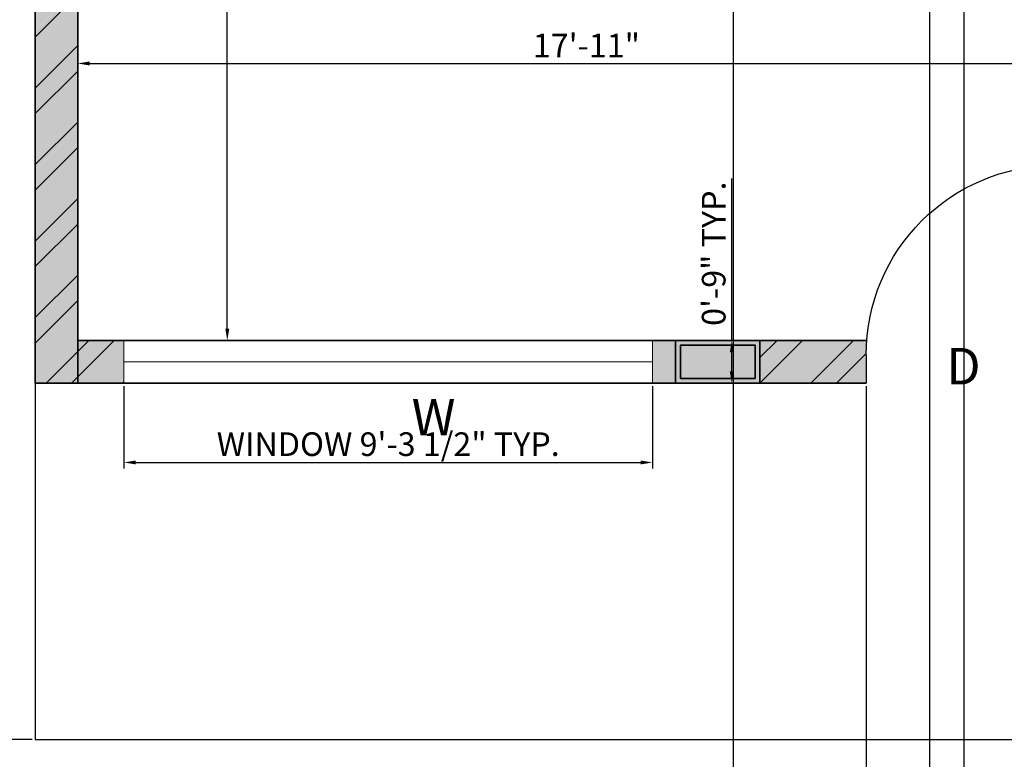
# Model space of a CAD drawing. Units: inches. Extents: x 1804 to 3296, y 909 to 2477.
# Tile 3 of 31: x 1922 to 2130, y 1059 to 1215. Entities that reach past the tile are written whole.
import ezdxf

# ---------------------------------------------------------------- set-up
doc = ezdxf.new("R2010")
doc.units = ezdxf.units.IN
for name, color, linetype, lineweight in [('A-ANNO-DIMS', 2, 'Continuous', 18), ('A-ANNO-TTLB', 156, 'Continuous', 35), ('A-WALL-PATT', 10, 'Continuous', 13), ('C-PROP', 7, 'Continuous', 25), ('DOOR', 30, 'Continuous', 25), ('TEXT', 190, 'Continuous', 18), ('WALL', 10, 'Continuous', 35), ('WIND', 130, 'Continuous', 18)]:
    doc.layers.add(name, color=color, linetype=linetype, lineweight=lineweight)
doc.styles.get("Standard").update_dxf_attribs({"font": 'arial.ttf'})
doc.dimstyles.new('ISO-25', dxfattribs={"dimtxt": 5, "dimasz": 2.5, "dimexe": 1.25, "dimexo": 0.625, "dimtad": 1, "dimdec": 0, "dimlunit": 4, "dimtxsty": 'Standard', "dimcen": 2.5, "dimadec": 0, "dimazin": 0, "dimtfac": 1, "dimtdec": 0, "dimtmove": 0, "dimatfit": 3, "dimfxl": 1, "dimarcsym": 0})

# ---------------------------------------------------------------- blocks, each defined once
blk = doc.blocks.new('*U2')
for p, q in [((0, 0), (0, -6)), ((40, 0), (40, -6))]:
    blk.add_line(p, q)
blk.add_lwpolyline([(0, 0), (0, 40), (1.75, 40), (1.75, 0)], close=True)
blk.add_arc((0, 0), 40, 0, 90)
blk = doc.blocks.new('*D21')
at = {"layer": 'A-ANNO-DIMS', "color": 0, "lineweight": -2, "transparency": 16777216}
for p, q in [((1935.21, 1539.88), (1967.44, 1539.88)), ((1966.19, 1149.57), (1966.19, 1537.38)), ((1935.21, 1147.07), (1967.44, 1147.07))]:
    blk.add_line(p, q, dxfattribs=at)
at = {"layer": 'A-ANNO-DIMS', "color": 0, "lineweight": 100, "transparency": 16777216}
for points in [[(1965.78, 1537.38), (1966.61, 1537.38), (1966.19, 1539.88)], [(1965.78, 1149.57), (1966.61, 1149.57), (1966.19, 1147.07)]]:
    blk.add_solid(points, dxfattribs=at)
at = {"layer": 'Defpoints', "color": 0, "lineweight": 100, "transparency": 16777216}
for p in [(1934.58, 1539.88), (1966.19, 1539.88), (1934.58, 1147.07)]:
    blk.add_point(p, dxfattribs=at)
at = {"layer": 'A-ANNO-DIMS', "color": 0, "transparency": 16777216, "insert": (1963.01, 1343.47), "char_height": 5, "attachment_point": 5, "rotation": 90}
blk.add_mtext('32\'-9"', dxfattribs=at)
blk = doc.blocks.new('*D22')
at = {"layer": 'A-ANNO-DIMS', "color": 0, "lineweight": -2, "transparency": 16777216}
for p, q in [((1934.58, 1147.69), (1934.58, 1206.88)), ((1937.08, 1205.63), (2147.08, 1205.63)), ((2149.58, 1147.69), (2149.58, 1206.88))]:
    blk.add_line(p, q, dxfattribs=at)
at = {"layer": 'A-ANNO-DIMS', "color": 0, "lineweight": 100, "transparency": 16777216}
for points in [[(1937.08, 1206.05), (1937.08, 1205.22), (1934.58, 1205.63)], [(2147.08, 1206.05), (2147.08, 1205.22), (2149.58, 1205.63)]]:
    blk.add_solid(points, dxfattribs=at)
at = {"layer": 'Defpoints', "color": 0, "lineweight": 100, "transparency": 16777216}
for p in [(2149.58, 1205.63), (1934.58, 1147.07), (2149.58, 1147.07)]:
    blk.add_point(p, dxfattribs=at)
at = {"layer": 'A-ANNO-DIMS', "color": 0, "transparency": 16777216, "insert": (2042.08, 1208.77), "char_height": 5, "attachment_point": 5}
blk.add_mtext('17\'-11"', dxfattribs=at)
blk = doc.blocks.new('WINDOW-PLAN-112IN')
blk.add_line((0, 4.5), (111.7, 4.5))
blk.add_lwpolyline([(0, 0), (111.7, 0), (111.7, 9), (0, 9)], close=True)
blk = doc.blocks.new('*D47')
at = {"layer": 'A-ANNO-DIMS', "color": 0, "lineweight": -2, "transparency": 16777216}
for p, q in [((1944.35, 1137.44), (1944.35, 1120.06)), ((2056.05, 1137.44), (2056.05, 1120.06)), ((1946.85, 1121.31), (2053.55, 1121.31))]:
    blk.add_line(p, q, dxfattribs=at)
at = {"layer": 'A-ANNO-DIMS', "color": 0, "lineweight": 100, "transparency": 16777216}
for points in [[(1946.85, 1121.73), (1946.85, 1120.9), (1944.35, 1121.31)], [(2053.55, 1121.73), (2053.55, 1120.9), (2056.05, 1121.31)]]:
    blk.add_solid(points, dxfattribs=at)
at = {"layer": 'Defpoints', "color": 0, "lineweight": 100, "transparency": 16777216}
for p in [(1944.35, 1138.07), (2056.05, 1138.07), (2056.05, 1121.31)]:
    blk.add_point(p, dxfattribs=at)
at = {"layer": 'A-ANNO-DIMS', "color": 0, "transparency": 16777216, "insert": (2000.2, 1124.53), "char_height": 5, "attachment_point": 5}
blk.add_mtext('WINDOW 9\'-3 1/2" TYP.', dxfattribs=at)
blk = doc.blocks.new('*D48')
at = {"layer": 'A-ANNO-DIMS', "color": 0, "lineweight": -2, "transparency": 16777216}
for p, q in [((2072.81, 1147.07), (2072.81, 1181.3)), ((2056.68, 1147.07), (2074.06, 1147.07)), ((2072.81, 1140.57), (2072.81, 1144.57)), ((2056.68, 1138.07), (2074.06, 1138.07))]:
    blk.add_line(p, q, dxfattribs=at)
at = {"layer": 'A-ANNO-DIMS', "color": 0, "lineweight": 100, "transparency": 16777216}
for points in [[(2072.39, 1144.57), (2073.22, 1144.57), (2072.81, 1147.07)], [(2072.39, 1140.57), (2073.22, 1140.57), (2072.81, 1138.07)]]:
    blk.add_solid(points, dxfattribs=at)
at = {"layer": 'Defpoints', "color": 0, "lineweight": 100, "transparency": 16777216}
for p in [(2056.05, 1147.07), (2072.81, 1147.07), (2056.05, 1138.07)]:
    blk.add_point(p, dxfattribs=at)
at = {"layer": 'A-ANNO-DIMS', "color": 0, "transparency": 16777216, "insert": (2069.63, 1165.43), "char_height": 5, "attachment_point": 5, "rotation": 90}
blk.add_mtext('0\'-9" TYP.', dxfattribs=at)
blk = doc.blocks.new('*D52')
at = {"layer": 'A-ANNO-DIMS', "color": 0, "lineweight": -2, "transparency": 16777216}
for p, q in [((1924.96, 1830.04), (1880.63, 1830.04)), ((1881.88, 1065.27), (1881.88, 1827.54)), ((1924.96, 1062.77), (1880.63, 1062.77))]:
    blk.add_line(p, q, dxfattribs=at)
at = {"layer": 'A-ANNO-DIMS', "color": 0, "lineweight": 100, "transparency": 16777216}
for points in [[(1881.47, 1827.54), (1882.3, 1827.54), (1881.88, 1830.04)], [(1881.47, 1065.27), (1882.3, 1065.27), (1881.88, 1062.77)]]:
    blk.add_solid(points, dxfattribs=at)
at = {"layer": 'Defpoints', "color": 0, "lineweight": 100, "transparency": 16777216}
for p in [(1881.88, 1830.04), (1925.58, 1830.04), (1925.58, 1062.77)]:
    blk.add_point(p, dxfattribs=at)
at = {"layer": 'A-ANNO-DIMS', "color": 0, "transparency": 16777216, "insert": (1878.67, 1446.4), "char_height": 5, "attachment_point": 5, "rotation": 90}
blk.add_mtext('63\'-11 1/2"', dxfattribs=at)
blk = doc.blocks.new('*D59')
at = {"layer": 'A-ANNO-DIMS', "color": 0, "lineweight": -2, "transparency": 16777216}
for p, q in [((2121.83, 1590.3), (2121.83, 975.89)), ((2161.83, 1590.3), (2161.83, 975.89)), ((2124.33, 977.14), (2159.33, 977.14))]:
    blk.add_line(p, q, dxfattribs=at)
at = {"layer": 'A-ANNO-DIMS', "color": 0, "lineweight": 100, "transparency": 16777216}
for points in [[(2124.33, 977.56), (2124.33, 976.72), (2121.83, 977.14)], [(2159.33, 977.56), (2159.33, 976.72), (2161.83, 977.14)]]:
    blk.add_solid(points, dxfattribs=at)
at = {"layer": 'Defpoints', "color": 0, "lineweight": 100, "transparency": 16777216}
for p in [(2121.83, 1590.92), (2161.83, 1590.92), (2161.83, 977.14)]:
    blk.add_point(p, dxfattribs=at)
at = {"layer": 'A-ANNO-DIMS', "color": 0, "transparency": 16777216, "insert": (2141.83, 980.32), "char_height": 5, "attachment_point": 5}
blk.add_mtext('3\'-4"', dxfattribs=at)
blk = doc.blocks.new('*D60')
at = {"layer": 'A-ANNO-DIMS', "color": 0, "lineweight": -2, "transparency": 16777216}
for p, q in [((2073.08, 1544.95), (2073.08, 975.89)), ((2114.58, 1543.75), (2114.58, 975.89)), ((2112.08, 977.14), (2075.58, 977.14))]:
    blk.add_line(p, q, dxfattribs=at)
at = {"layer": 'A-ANNO-DIMS', "color": 0, "lineweight": 100, "transparency": 16777216}
for points in [[(2075.58, 977.56), (2075.58, 976.72), (2073.08, 977.14)], [(2112.08, 977.56), (2112.08, 976.72), (2114.58, 977.14)]]:
    blk.add_solid(points, dxfattribs=at)
at = {"layer": 'Defpoints', "color": 0, "lineweight": 100, "transparency": 16777216}
for p in [(2073.08, 1545.58), (2114.58, 1544.38), (2073.08, 977.14)]:
    blk.add_point(p, dxfattribs=at)
at = {"layer": 'A-ANNO-DIMS', "color": 0, "transparency": 16777216, "insert": (2093.83, 980.35), "char_height": 5, "attachment_point": 5}
blk.add_mtext('3\'-5 1/2"', dxfattribs=at)
blk = doc.blocks.new('*D61')
at = {"layer": 'A-ANNO-DIMS', "color": 0, "lineweight": -2, "transparency": 16777216}
for p, q in [((2101.21, 1137.44), (2101.21, 975.89)), ((2141.21, 1137.44), (2141.21, 975.89)), ((2103.71, 977.14), (2138.71, 977.14))]:
    blk.add_line(p, q, dxfattribs=at)
at = {"layer": 'A-ANNO-DIMS', "color": 0, "lineweight": 100, "transparency": 16777216}
for points in [[(2103.71, 977.56), (2103.71, 976.72), (2101.21, 977.14)], [(2138.71, 977.56), (2138.71, 976.72), (2141.21, 977.14)]]:
    blk.add_solid(points, dxfattribs=at)
at = {"layer": 'Defpoints', "color": 0, "lineweight": 100, "transparency": 16777216}
for p in [(2101.21, 1138.07), (2141.21, 1138.07), (2141.21, 977.14)]:
    blk.add_point(p, dxfattribs=at)
at = {"layer": 'A-ANNO-DIMS', "color": 0, "transparency": 16777216, "insert": (2121.21, 980.32), "char_height": 5, "attachment_point": 5}
blk.add_mtext('3\'-4"', dxfattribs=at)

msp = doc.modelspace()

# ---------------------------------------------------------------- hatches: boundary and pattern name
at = {"layer": 'A-ANNO-TTLB'}
h = msp.add_hatch(color=256, dxfattribs=at)
h.dxf.hatch_style = 1
h.paths.add_polyline_path([(3294.53, 2476.54), (1803.79, 2476.54), (1805.43, 909.47), (3296.17, 909.47)])
h.paths.add_polyline_path([(1811, 914.33), (1812.79, 2467.54), (3285.53, 2467.54), (3283.74, 914.33)], flags=16)
h.paths.add_polyline_path([(1925.58, 1062.77), (1925.58, 1138.07), (1925.58, 1539.88), (1925.58, 1793.38), (1925.58, 1830.04), (2325.54, 1830.04), (2325.54, 1793.38), (2325.54, 1586.42), (2325.54, 1138.07), (2325.54, 1062.77)], flags=0)
h.paths.add_polyline_path([(1997.22, 1029.4), (2008.85, 1037.96), (2008.85, 1020.84)], flags=0)
h.paths.add_polyline_path([(1934.58, 1138.07), (1934.58, 1147.07), (2078.77, 1147.07), (2078.77, 1138.07), (2060.94, 1138.07)], flags=0)
h.paths.add_polyline_path([(1944.35, 1138.07), (1944.35, 1147.07), (2056.05, 1147.07), (2056.05, 1138.07)], flags=0)
h.paths.add_polyline_path([(2222.24, 1037.96), (2233.87, 1029.4), (2222.24, 1020.84)], flags=0)
h.paths.add_polyline_path([(2061.94, 1139.07), (2061.94, 1146.07), (2077.77, 1146.07), (2077.77, 1139.07)], flags=0)
h.paths.add_polyline_path([(2149.58, 1138.07), (2149.58, 1269.44), (2158.58, 1269.44), (2158.58, 1326.69), (2149.58, 1326.69), (2149.58, 1340.94), (2139.6, 1340.94), (2139.6, 1434.25), (2149.58, 1434.25), (2149.58, 1447.36), (2158.58, 1447.36), (2158.58, 1423.87), (2158.58, 1408.06), (2198.46, 1408.06), (2198.46, 1412.56), (2282.65, 1412.56), (2282.65, 1465.94), (2316.54, 1465.94), (2316.54, 1590.92), (2192.86, 1590.92), (2192.86, 1595.3), (2291.17, 1595.3), (2291.17, 1590.92), (2316.54, 1590.92), (2316.54, 1784.38), (2300.24, 1784.38), (2300.24, 1757.47), (2268, 1757.47), (2268, 1681.04), (2180.87, 1681.04), (2180.87, 1757.47), (2148.63, 1757.47), (2148.63, 1784.38), (2119.08, 1784.38), (2119.08, 1585.58), (2114.58, 1585.58), (2114.58, 1784.38), (2064.11, 1784.38), (2046.28, 1784.38), (2046.28, 1760.38), (1958.58, 1760.38), (1958.58, 1664.38), (1934.58, 1664.38), (1934.58, 1784.38), (1934.58, 1793.38), (2046.28, 1793.38), (2064.11, 1793.38), (2119.08, 1793.38), (2230.78, 1793.38), (2230.78, 1784.38), (2268, 1784.38), (2300.24, 1784.38), (2316.54, 1784.38), (2316.54, 1590.92), (2316.54, 1373.73), (2316.54, 1138.07)], flags=0)
h.paths.add_polyline_path([(2209.19, 1166.63), (2209.19, 1175.63), (2158.58, 1175.63), (2209.19, 1223.63), (2209.19, 1231.63), (2183.88, 1231.63), (2183.88, 1301.66), (2242.59, 1301.66), (2242.59, 1326.69), (2316.54, 1326.69), (2272.59, 1271.63), (2272.59, 1223.63), (2316.54, 1175.63), (2272.59, 1175.63), (2272.59, 1166.63)], flags=0)
h.paths.add_polyline_path([(1947.77, 1345.22), (1947.77, 1457.48), (1991.2, 1457.48), (1991.2, 1451.7), (1991.2, 1352.18), (1991.2, 1345.22)], flags=0)
h.paths.add_polyline_path([(2209.19, 1271.63), (2262.59, 1271.63), (2262.59, 1311.85), (2272.59, 1301.66), (2272.59, 1271.63), (2269.92, 1269.63), (2270.59, 1269.63), (2270.59, 1225.63), (2211.19, 1225.63), (2211.19, 1269.63), (2211.86, 1269.63)], flags=0)
h.paths.add_polyline_path([(2000.34, 1378.21), (2000.34, 1429.71), (2025.22, 1429.71), (2025.22, 1378.21)], flags=0)
h.paths.add_polyline_path([(2001.34, 1379.21), (2001.34, 1428.71), (2024.22, 1428.71), (2024.22, 1379.21)], flags=0)
h.paths.add_polyline_path([(2012.34, 1390.21), (2012.34, 1417.71), (2013.22, 1417.71), (2013.22, 1390.21)], flags=0)
h.paths.add_polyline_path([(2237.56, 1331.19), (2237.56, 1340.18), (2238.62, 1340.18), (2238.62, 1386.84), (2241.04, 1386.84), (2242.06, 1386.84), (2242.06, 1408.06), (2316.54, 1331.19)], flags=0)
h.paths.add_polyline_path([(1953.73, 1464.35), (1953.73, 1498.59), (1981.74, 1498.59), (1981.74, 1464.35)], flags=0)
h.paths.add_polyline_path([(1987.63, 1462.08), (1987.63, 1500.95), (2104.07, 1500.95), (2104.07, 1462.08), (2099.27, 1462.08), (1993.6, 1462.08)], flags=0)
h.paths.add_polyline_path([(1956.06, 1481.47, -1), (1979.41, 1481.47, -1)], flags=0)
edge = h.paths.add_edge_path(flags=0)
edge.add_ellipse((2299.53, 1438.37), major_axis=(0.31, 21.36), ratio=0.670333, start_angle=0, end_angle=360)
h.paths.add_polyline_path([(2297.39, 1438.37, -1), (2301.67, 1438.37, -1)], flags=0)
h.paths.add_polyline_path([(2591.54, 1163.23), (2591.54, 1179.38), (2591.54, 1379.68), (2591.54, 1395.84), (2734.5, 1395.84), (2734.5, 1379.68), (2734.5, 1179.38), (2734.5, 1163.23)], flags=0)
h.paths.add_polyline_path([(2592.54, 1164.23), (2592.54, 1166.23), (2733.5, 1166.23), (2733.5, 1164.23)], flags=0)
h.paths.add_polyline_path([(2592.54, 1180.38), (2592.54, 1378.68), (2733.5, 1378.68), (2733.5, 1180.38)], flags=0)
h.paths.add_polyline_path([(2593.54, 1181.38), (2593.54, 1377.68), (2732.5, 1377.68), (2732.5, 1181.38)], flags=0)
h.paths.add_polyline_path([(2594.54, 1182.38), (2594.54, 1376.68), (2731.5, 1376.68), (2731.5, 1182.38)], flags=0)
h.paths.add_polyline_path([(1936.95, 1697.46), (1936.95, 1736.46), (1955.41, 1736.46), (1955.41, 1697.46)], flags=0)
h.paths.add_polyline_path([(1938.48, 1718.36), (1938.48, 1734.92), (1953.65, 1734.92), (1953.65, 1718.36)], flags=0)
h.paths.add_polyline_path([(1944.75, 1726.64, -1), (1947.37, 1726.64, -1)], flags=0)
h.paths.add_polyline_path([(2592.54, 1394.84), (2733.5, 1394.84), (2733.5, 1392.84), (2592.54, 1392.84)], flags=0)
h.paths.add_polyline_path([(1976.61, 1762.5), (1976.61, 1781.44), (2012.79, 1781.44), (2012.79, 1762.5)], flags=0)
h.paths.add_polyline_path([(1979.57, 1771.97, -1), (1991.39, 1771.97, -1)], flags=0)
h.paths.add_polyline_path([(1995.36, 1771.97, -1), (2007.18, 1771.97, -1)], flags=0)
h.paths.add_polyline_path([(2251.51, 1744.53), (2268, 1730.05), (2251.51, 1730.05)], flags=0)
h.paths.add_polyline_path([(2047.28, 1785.38), (2047.28, 1792.38), (2063.11, 1792.38), (2063.11, 1785.38)], flags=0)
h.paths.add_polyline_path([(2155.08, 1770.92, -1), (2174.42, 1770.92, -1)], flags=0)
h.paths.add_polyline_path([(2188.59, 1758.27), (2188.59, 1772.81), (2222.3, 1772.81), (2222.3, 1758.27)], flags=0)
h.paths.add_polyline_path([(2223.97, 1758.27), (2223.97, 1772.81), (2257.68, 1772.81), (2257.68, 1758.27)], flags=0)
h.paths.add_polyline_path([(2274.45, 1770.92, -1), (2293.8, 1770.92, -1)], flags=0)
h.paths.add_polyline_path([(2591.54, 1582.09), (2591.54, 1782.39), (2734.5, 1782.39), (2734.5, 1582.09)], flags=0)
h.paths.add_polyline_path([(2592.54, 1583.09), (2592.54, 1781.39), (2733.5, 1781.39), (2733.5, 1583.09)], flags=0)
h.paths.add_polyline_path([(2593.54, 1584.09), (2593.54, 1780.39), (2732.5, 1780.39), (2732.5, 1584.09)], flags=0)
h.paths.add_polyline_path([(2594.54, 1585.09), (2594.54, 1779.39), (2731.5, 1779.39), (2731.5, 1585.09)], flags=0)
h.paths.add_polyline_path([(1922.17, 1978.79), (1922.17, 2295.08), (1922.17, 2296.08), (2115.67, 2296.08), (2115.67, 2384.31), (2115.67, 2385.31), (2322.12, 2385.31), (2323.12, 2385.31), (2323.12, 1979.79), (2323.12, 1978.79), (1923.17, 1978.79)], flags=0)
h.paths.add_polyline_path([(1922.17, 1978.79), (1922.17, 2051.31), (1922.17, 2214.86), (1922.17, 2296.08), (2115.67, 2296.08), (2115.67, 2385.31), (2323.12, 2385.31), (2323.12, 2280.42), (2323.12, 1978.79), (2115.67, 1978.79)], flags=0)
h.paths.add_polyline_path([(1923.17, 1979.79), (1923.17, 2050.31), (2115.67, 2050.31), (2115.67, 2051.31), (1923.17, 2051.31), (1923.17, 2213.86), (1923.17, 2214.86), (1923.17, 2295.08), (1990.02, 2295.08), (1990.02, 2214.86), (1991.02, 2214.86), (1991.02, 2295.08), (2115.67, 2295.08), (2115.67, 1979.79), (2116.67, 1979.79), (2116.67, 2304.18), (2116.67, 2384.31), (2322.12, 2384.31), (2322.12, 2280.42), (2322.12, 1979.79), (2115.67, 1979.79)], flags=0)
h.paths.add_polyline_path([(2972.46, 1192.5), (2972.46, 1196.92), (2995.47, 1196.92), (2995.47, 1255.47), (2995.09, 1255.47), (2987.42, 1249.39), (2980.08, 1255.47), (2978.05, 1255.47), (2978.05, 1257.24), (2995.47, 1257.24), (2995.47, 1261.58), (3015.37, 1261.58), (3015.37, 1333.28), (3015.37, 1414.4), (3032.82, 1414.4), (3032.82, 1333.28), (3032.82, 1261.58), (3052.66, 1261.58), (3052.66, 1255.47), (3079.86, 1255.47), (3078.72, 1254.57), (3081.47, 1252.29), (3078.56, 1249.99), (3075.81, 1252.26), (3072.57, 1249.69), (3070.36, 1251.52), (3067.67, 1249.39), (3060.34, 1255.47), (3052.66, 1255.47), (3052.66, 1196.92), (3054.58, 1196.92), (3074, 1196.92), (3074, 1192.5), (3052.66, 1192.5), (2995.47, 1192.5)], flags=0)
h.paths.add_polyline_path([(2490.75, 1979.27), (2490.75, 1980.27), (2596.87, 1980.27), (2596.87, 2051.8), (2596.87, 2052.8), (2596.87, 2216.35), (2596.87, 2297.57), (2717.32, 2297.57), (2710.57, 2305.62), (2724.07, 2305.62), (2717.32, 2297.57), (2782.37, 2297.57), (2782.37, 2395.8), (3006.82, 2395.8), (3006.82, 1981.27), (3093.73, 1981.27), (3093.73, 1980.27), (3047.51, 1980.27), (3046.37, 1979.37), (3049.11, 1977.1), (3046.2, 1974.79), (3043.46, 1977.07), (3040.21, 1974.49), (3038, 1976.32), (3035.32, 1974.2), (3027.98, 1980.27), (2871.83, 1980.27), (2871.83, 1981.27), (2791.37, 1981.27), (2791.37, 2050.8), (2597.87, 2050.8), (2597.87, 1980.27), (2597.87, 1979.27), (2546.27, 1979.27), (2545.12, 1978.37), (2547.87, 1976.1), (2544.96, 1973.79), (2542.22, 1976.07), (2538.97, 1973.49), (2536.76, 1975.32), (2534.07, 1973.2), (2526.74, 1979.27)], flags=0)
h.paths.add_polyline_path([(2597.87, 2051.8), (2606.87, 2051.8), (2606.87, 2258.39), (2597.87, 2258.39), (2597.87, 2296.57), (2606.87, 2296.57), (2606.87, 2262.39), (2782.37, 2262.39), (2782.37, 2296.57), (2790.37, 2296.57), (2790.37, 2262.39), (2791.37, 2262.39), (2791.37, 2305.67), (2791.37, 2385.8), (2996.82, 2385.8), (2996.82, 2339.85), (3006.82, 2339.85), (3006.82, 2250.12), (2997.82, 2250.12), (2997.82, 1981.27), (2996.82, 1981.27), (2872.83, 1981.27), (2872.83, 1991.8), (2871.83, 1991.8), (2871.83, 2050.8), (2790.37, 2050.8), (2597.87, 2050.8)], flags=0)
h.paths.add_polyline_path([(2179.93, 2153.92), (2179.93, 2353.97), (2259.98, 2353.97), (2259.98, 2153.92)], flags=0)
h.paths.add_polyline_path([(2180.93, 2154.92), (2180.93, 2352.97), (2258.98, 2352.97), (2258.98, 2154.92)], flags=0)
h.paths.add_polyline_path([(2960.87, 1608.49), (2960.87, 1753.62), (3070.9, 1753.62), (3070.9, 1608.49)], flags=0)
h.paths.add_polyline_path([(2961.87, 1609.49), (2961.87, 1752.62), (3069.9, 1752.62), (3069.9, 1609.49)], flags=0)
h.paths.add_polyline_path([(2962.87, 1610.49), (2962.87, 1751.62), (3068.9, 1751.62), (3068.9, 1610.49)], flags=0)
h.paths.add_polyline_path([(2963.87, 1611.49), (2963.87, 1750.62), (3067.9, 1750.62), (3067.9, 1611.49)], flags=0)
h.paths.add_polyline_path([(2782.37, 2051.8), (2782.37, 2216.32), (2791.37, 2216.32), (2791.37, 2051.8), (2872.83, 2051.8), (2872.83, 2068.56), (2884.67, 2068.56), (2884.67, 2085.33), (2896.51, 2085.33), (2896.51, 2102.09), (2908.36, 2102.09), (2908.36, 2118.85), (2920.2, 2118.85), (2920.2, 2135.62), (2932.05, 2135.62), (2932.05, 2145.3), (2925.08, 2145.3), (2925.08, 2203.2), (2996.82, 2203.2), (2996.82, 2145.3), (2953.82, 2145.3), (2872.83, 2051.8), (2790.37, 2051.8)], flags=0)
h.paths.add_polyline_path([(2717.32, 2238.65), (2710.57, 2246.7), (2724.07, 2246.7)], flags=0)
h.paths.add_polyline_path([(2003.09, 1122.79), (2017.16, 1122.79), (2017.16, 1138.74), (2003.09, 1138.74)], flags=8)
h.paths.add_polyline_path([(2174.76, 1792.72), (2188.83, 1792.72), (2188.83, 1808.66), (2174.76, 1808.66)], flags=8)
h.paths.add_polyline_path([(1987.95, 1792.51), (2002.02, 1792.51), (2002.02, 1808.45), (1987.95, 1808.45)], flags=8)
h.paths.add_polyline_path([(2148.79, 1289.26), (2160.46, 1289.26), (2160.46, 1305.2), (2148.79, 1305.2)], flags=8)
h.paths.add_polyline_path([(2115.36, 1133.57), (2127.04, 1133.57), (2127.04, 1149.51), (2115.36, 1149.51)], flags=8)
h.paths.add_polyline_path([(2237.58, 1421.48), (2249.25, 1421.48), (2249.25, 1437.43), (2237.58, 1437.43)], flags=8)
h.paths.add_polyline_path([(2134.99, 1584.32), (2146.66, 1584.32), (2146.66, 1600.26), (2134.99, 1600.26)], flags=8)
h.paths.add_polyline_path([(2101.95, 1557.31), (2113.62, 1557.31), (2113.62, 1573.25), (2101.95, 1573.25)], flags=8)
h.paths.add_polyline_path([(2937.85, 1156.77), (3120.41, 1156.77), (3120.41, 1185.72), (2937.85, 1185.72)], flags=8)
h.paths.add_polyline_path([(2980.71, 1786.71), (3050.06, 1786.71), (3050.06, 1802.66), (2980.71, 1802.66)], flags=8)
h.paths.add_polyline_path([(2869.28, 1661.96), (2938.62, 1661.96), (2938.62, 1690.8), (2869.28, 1690.8)], flags=8)
h.paths.add_polyline_path([(3092.27, 1674.86), (3161.62, 1674.86), (3161.62, 1690.8), (3092.27, 1690.8)], flags=8)
h.paths.add_polyline_path([(2980.71, 1674.86), (3050.06, 1674.86), (3050.06, 1690.8), (2980.71, 1690.8)], flags=8)
h.paths.add_polyline_path([(2649.07, 1678.23), (2674.53, 1678.23), (2674.53, 1714.76), (2649.07, 1714.76)], flags=8)
h.paths.add_polyline_path([(2530.84, 1981.63), (2549.13, 1981.63), (2549.13, 1997.57), (2530.84, 1997.57)], flags=8)
h.paths.add_polyline_path([(3031.29, 1981.77), (3049.58, 1981.77), (3049.58, 1997.71), (3031.29, 1997.71)], flags=8)
h.paths.add_polyline_path([(2715.38, 1911.9), (2851.54, 1911.9), (2851.54, 1940.85), (2715.38, 1940.85)], flags=8)
h.paths.add_polyline_path([(2015.23, 1927.36), (2205.42, 1927.36), (2205.42, 1956.3), (2015.23, 1956.3)], flags=8)
h.paths.add_polyline_path([(2671.84, 2057.84), (2702.75, 2057.84), (2702.75, 2073.79), (2671.84, 2073.79)], flags=8)
h.paths.add_polyline_path([(2678.5, 2316.52), (2765.26, 2316.52), (2765.26, 2332.46), (2678.5, 2332.46)], flags=8)
h.paths.add_polyline_path([(2678.48, 2271.96), (2736.41, 2271.96), (2736.41, 2287.9), (2678.48, 2287.9)], flags=8)
h.paths.add_polyline_path([(2019.2, 972.79), (2243.21, 972.79), (2243.21, 1001.74), (2019.2, 1001.74)], flags=8)
h.paths.add_polyline_path([(2097.06, 1021.56), (2132.16, 1021.56), (2132.16, 1037.51), (2097.06, 1037.51)], flags=8)
h.paths.add_polyline_path([(2182.47, 1360.48), (2207.35, 1360.48), (2207.35, 1376.42), (2182.47, 1376.42)], flags=8)
h.paths.add_polyline_path([(2261.12, 1361.77), (2295.01, 1361.77), (2295.01, 1377.71), (2261.12, 1377.71)], flags=8)
h.paths.add_polyline_path([(2245.75, 1511.51), (2278.44, 1511.51), (2278.44, 1527.46), (2245.75, 1527.46)], flags=8)
h.paths.add_polyline_path([(1991.16, 1296.29), (2060.51, 1296.29), (2060.51, 1312.23), (1991.16, 1312.23)], flags=8)
h.paths.add_polyline_path([(2187, 1651.35), (2246.71, 1651.35), (2246.71, 1667.29), (2187, 1667.29)], flags=8)
h.paths.add_polyline_path([(1976.49, 1684.81), (2068.63, 1684.81), (2068.63, 1700.76), (1976.49, 1700.76)], flags=8)
at = {"layer": 'A-WALL-PATT'}
h = msp.add_hatch(color=256, dxfattribs=at)
h.dxf.hatch_style = 1
h.paths.add_polyline_path([(2119.08, 1544.38), (1925.58, 1544.38), (1925.58, 1539.88), (2119.08, 1539.88)])
h.paths.add_polyline_path([(2119.08, 1545.58), (2114.58, 1545.58), (2114.58, 1544.38), (2119.08, 1544.38)])
h.paths.add_polyline_path([(1965.87, 1658.79), (1965.87, 1679.09), (1955.57, 1679.09), (1955.57, 1658.79)], flags=9)
h.paths.add_polyline_path([(2293.18, 1677.29), (2293.18, 1697.58), (2282.88, 1697.58), (2282.88, 1677.29)], flags=9)
h.paths.add_polyline_path([(2271.13, 1545.23), (2287.53, 1545.23), (2287.53, 1555.53), (2271.13, 1555.53)], flags=9)
h.paths.add_polyline_path([(2303.26, 1488.52), (2303.26, 1508.82), (2292.95, 1508.82), (2292.95, 1488.52)], flags=9)
h.paths.add_polyline_path([(2271.13, 1393.15), (2287.53, 1393.15), (2287.53, 1403.45), (2271.13, 1403.45)], flags=9)
h.paths.add_polyline_path([(2306.48, 1361.45), (2306.48, 1377.86), (2296.18, 1377.86), (2296.18, 1361.45)], flags=9)
h.paths.add_polyline_path([(2174.54, 1361.45), (2174.54, 1377.86), (2164.23, 1377.86), (2164.23, 1361.45)], flags=9)
h.paths.add_polyline_path([(1968.21, 1333.34), (1968.21, 1353.64), (1957.91, 1353.64), (1957.91, 1333.34)], flags=9)
h.paths.add_polyline_path([(2003.09, 1122.79), (2017.16, 1122.79), (2017.16, 1138.74), (2003.09, 1138.74)], flags=9)
h.paths.add_polyline_path([(2174.76, 1792.72), (2188.83, 1792.72), (2188.83, 1808.66), (2174.76, 1808.66)], flags=9)
h.paths.add_polyline_path([(1987.95, 1792.51), (2002.02, 1792.51), (2002.02, 1808.45), (1987.95, 1808.45)], flags=9)
h.paths.add_polyline_path([(2148.79, 1289.26), (2160.46, 1289.26), (2160.46, 1305.2), (2148.79, 1305.2)], flags=9)
h.paths.add_polyline_path([(2115.36, 1133.57), (2127.04, 1133.57), (2127.04, 1149.51), (2115.36, 1149.51)], flags=9)
h.paths.add_polyline_path([(2237.58, 1421.48), (2249.25, 1421.48), (2249.25, 1437.43), (2237.58, 1437.43)], flags=9)
h.paths.add_polyline_path([(2134.99, 1584.32), (2146.66, 1584.32), (2146.66, 1600.26), (2134.99, 1600.26)], flags=9)
h.paths.add_polyline_path([(2101.95, 1557.31), (2113.62, 1557.31), (2113.62, 1573.25), (2101.95, 1573.25)], flags=9)
h.paths.add_polyline_path([(2937.85, 1156.77), (3120.41, 1156.77), (3120.41, 1185.72), (2937.85, 1185.72)], flags=9)
h.paths.add_polyline_path([(2980.71, 1786.71), (3050.06, 1786.71), (3050.06, 1802.66), (2980.71, 1802.66)], flags=9)
h.paths.add_polyline_path([(2869.28, 1661.96), (2938.62, 1661.96), (2938.62, 1690.8), (2869.28, 1690.8)], flags=9)
h.paths.add_polyline_path([(3092.27, 1674.86), (3161.62, 1674.86), (3161.62, 1690.8), (3092.27, 1690.8)], flags=9)
h.paths.add_polyline_path([(2980.71, 1674.86), (3050.06, 1674.86), (3050.06, 1690.8), (2980.71, 1690.8)], flags=9)
h.paths.add_polyline_path([(2649.07, 1678.23), (2674.53, 1678.23), (2674.53, 1714.76), (2649.07, 1714.76)], flags=9)
h.paths.add_polyline_path([(2530.84, 1981.63), (2549.13, 1981.63), (2549.13, 1997.57), (2530.84, 1997.57)], flags=9)
h.paths.add_polyline_path([(3031.29, 1981.77), (3049.58, 1981.77), (3049.58, 1997.71), (3031.29, 1997.71)], flags=9)
h.paths.add_polyline_path([(2715.38, 1911.9), (2851.54, 1911.9), (2851.54, 1940.85), (2715.38, 1940.85)], flags=9)
h.paths.add_polyline_path([(2015.23, 1927.36), (2205.42, 1927.36), (2205.42, 1956.3), (2015.23, 1956.3)], flags=9)
h.paths.add_polyline_path([(2671.84, 2057.84), (2702.75, 2057.84), (2702.75, 2073.79), (2671.84, 2073.79)], flags=9)
h.paths.add_polyline_path([(2678.5, 2316.52), (2765.26, 2316.52), (2765.26, 2332.46), (2678.5, 2332.46)], flags=9)
h.paths.add_polyline_path([(2678.48, 2271.96), (2736.41, 2271.96), (2736.41, 2287.9), (2678.48, 2287.9)], flags=9)
h.paths.add_polyline_path([(2019.2, 972.79), (2243.21, 972.79), (2243.21, 1001.74), (2019.2, 1001.74)], flags=9)
h.paths.add_polyline_path([(2097.06, 1021.56), (2132.16, 1021.56), (2132.16, 1037.51), (2097.06, 1037.51)], flags=9)
h.paths.add_polyline_path([(2182.47, 1360.48), (2207.35, 1360.48), (2207.35, 1376.42), (2182.47, 1376.42)], flags=9)
h.paths.add_polyline_path([(2261.12, 1361.77), (2295.01, 1361.77), (2295.01, 1377.71), (2261.12, 1377.71)], flags=9)
h.paths.add_polyline_path([(2245.75, 1511.51), (2278.44, 1511.51), (2278.44, 1527.46), (2245.75, 1527.46)], flags=9)
h.paths.add_polyline_path([(1991.16, 1296.29), (2060.51, 1296.29), (2060.51, 1312.23), (1991.16, 1312.23)], flags=9)
h.paths.add_polyline_path([(2187, 1651.35), (2246.71, 1651.35), (2246.71, 1667.29), (2187, 1667.29)], flags=9)
h.paths.add_polyline_path([(1976.49, 1684.81), (2068.63, 1684.81), (2068.63, 1700.76), (1976.49, 1700.76)], flags=9)
h = msp.add_hatch(color=256, dxfattribs=at)
h.dxf.hatch_style = 1
h.paths.add_polyline_path([(2149.58, 1147.07), (2141.21, 1147.07), (2141.21, 1144.07), (2141.21, 1138.07), (2149.58, 1138.07)])
h.paths.add_polyline_path([(2101.21, 1144.07, -0.01877), (2101.32, 1147.07), (2078.77, 1147.07), (2078.77, 1138.07), (2101.21, 1138.07)])
h.paths.add_polyline_path([(2060.94, 1147.07), (2056.05, 1147.07), (2056.05, 1138.07), (2060.94, 1138.07)])
h.paths.add_polyline_path([(1944.35, 1147.07), (1934.58, 1147.07), (1934.58, 1138.07), (1944.35, 1138.07)])
h.paths.add_polyline_path([(2158.58, 1269.44), (2149.58, 1269.44), (2149.58, 1138.07), (2158.58, 1138.07)])
h.paths.add_polyline_path([(2003.09, 1122.79), (2017.16, 1122.79), (2017.16, 1138.74), (2003.09, 1138.74)], flags=9)
h.paths.add_polyline_path([(2174.76, 1792.72), (2188.83, 1792.72), (2188.83, 1808.66), (2174.76, 1808.66)], flags=9)
h.paths.add_polyline_path([(1987.95, 1792.51), (2002.02, 1792.51), (2002.02, 1808.45), (1987.95, 1808.45)], flags=9)
h.paths.add_polyline_path([(2148.79, 1289.26), (2160.46, 1289.26), (2160.46, 1305.2), (2148.79, 1305.2)], flags=9)
h.paths.add_polyline_path([(2115.36, 1133.57), (2127.04, 1133.57), (2127.04, 1149.51), (2115.36, 1149.51)], flags=9)
h.paths.add_polyline_path([(2237.58, 1421.48), (2249.25, 1421.48), (2249.25, 1437.43), (2237.58, 1437.43)], flags=9)
h.paths.add_polyline_path([(2134.99, 1584.32), (2146.66, 1584.32), (2146.66, 1600.26), (2134.99, 1600.26)], flags=9)
h.paths.add_polyline_path([(2101.95, 1557.31), (2113.62, 1557.31), (2113.62, 1573.25), (2101.95, 1573.25)], flags=9)
h.paths.add_polyline_path([(2937.85, 1156.77), (3120.41, 1156.77), (3120.41, 1185.72), (2937.85, 1185.72)], flags=9)
h.paths.add_polyline_path([(2980.71, 1786.71), (3050.06, 1786.71), (3050.06, 1802.66), (2980.71, 1802.66)], flags=9)
h.paths.add_polyline_path([(2869.28, 1661.96), (2938.62, 1661.96), (2938.62, 1690.8), (2869.28, 1690.8)], flags=9)
h.paths.add_polyline_path([(3092.27, 1674.86), (3161.62, 1674.86), (3161.62, 1690.8), (3092.27, 1690.8)], flags=9)
h.paths.add_polyline_path([(2980.71, 1674.86), (3050.06, 1674.86), (3050.06, 1690.8), (2980.71, 1690.8)], flags=9)
h.paths.add_polyline_path([(2649.07, 1678.23), (2674.53, 1678.23), (2674.53, 1714.76), (2649.07, 1714.76)], flags=9)
h.paths.add_polyline_path([(2530.84, 1981.63), (2549.13, 1981.63), (2549.13, 1997.57), (2530.84, 1997.57)], flags=9)
h.paths.add_polyline_path([(3031.29, 1981.77), (3049.58, 1981.77), (3049.58, 1997.71), (3031.29, 1997.71)], flags=9)
h.paths.add_polyline_path([(2715.38, 1911.9), (2851.54, 1911.9), (2851.54, 1940.85), (2715.38, 1940.85)], flags=9)
h.paths.add_polyline_path([(2015.23, 1927.36), (2205.42, 1927.36), (2205.42, 1956.3), (2015.23, 1956.3)], flags=9)
h.paths.add_polyline_path([(2671.84, 2057.84), (2702.75, 2057.84), (2702.75, 2073.79), (2671.84, 2073.79)], flags=9)
h.paths.add_polyline_path([(2678.5, 2316.52), (2765.26, 2316.52), (2765.26, 2332.46), (2678.5, 2332.46)], flags=9)
h.paths.add_polyline_path([(2678.48, 2271.96), (2736.41, 2271.96), (2736.41, 2287.9), (2678.48, 2287.9)], flags=9)
h.paths.add_polyline_path([(2019.2, 972.79), (2243.21, 972.79), (2243.21, 1001.74), (2019.2, 1001.74)], flags=9)
h.paths.add_polyline_path([(2097.06, 1021.56), (2132.16, 1021.56), (2132.16, 1037.51), (2097.06, 1037.51)], flags=9)
h.paths.add_polyline_path([(2182.47, 1360.48), (2207.35, 1360.48), (2207.35, 1376.42), (2182.47, 1376.42)], flags=9)
h.paths.add_polyline_path([(2261.12, 1361.77), (2295.01, 1361.77), (2295.01, 1377.71), (2261.12, 1377.71)], flags=9)
h.paths.add_polyline_path([(2245.75, 1511.51), (2278.44, 1511.51), (2278.44, 1527.46), (2245.75, 1527.46)], flags=9)
h.paths.add_polyline_path([(1991.16, 1296.29), (2060.51, 1296.29), (2060.51, 1312.23), (1991.16, 1312.23)], flags=9)
h.paths.add_polyline_path([(2187, 1651.35), (2246.71, 1651.35), (2246.71, 1667.29), (2187, 1667.29)], flags=9)
h.paths.add_polyline_path([(1976.49, 1684.81), (2068.63, 1684.81), (2068.63, 1700.76), (1976.49, 1700.76)], flags=9)
h = msp.add_hatch(color=256, dxfattribs=at)
h.dxf.hatch_style = 1
h.paths.add_polyline_path([(2158.58, 1275.49), (2155.29, 1275.49), (2149.58, 1275.49), (2149.58, 1269.44), (2158.58, 1269.44)])
h.paths.add_polyline_path([(2158.58, 1326.69), (2149.58, 1326.69), (2149.58, 1319.33), (2155.29, 1319.33), (2158.58, 1319.33)])
h.paths.add_polyline_path([(2158.58, 1402.2), (2158.58, 1423.87), (2158.58, 1447.36), (2149.58, 1447.36), (2149.58, 1423.87), (2149.58, 1340.94), (2149.58, 1326.69), (2158.58, 1326.69), (2158.58, 1354.23)])
h.paths.add_polyline_path([(1965.87, 1658.79), (1965.87, 1679.09), (1955.57, 1679.09), (1955.57, 1658.79)], flags=9)
h.paths.add_polyline_path([(2293.18, 1677.29), (2293.18, 1697.58), (2282.88, 1697.58), (2282.88, 1677.29)], flags=9)
h.paths.add_polyline_path([(2271.13, 1545.23), (2287.53, 1545.23), (2287.53, 1555.53), (2271.13, 1555.53)], flags=9)
h.paths.add_polyline_path([(2303.26, 1488.52), (2303.26, 1508.82), (2292.95, 1508.82), (2292.95, 1488.52)], flags=9)
h.paths.add_polyline_path([(2271.13, 1393.15), (2287.53, 1393.15), (2287.53, 1403.45), (2271.13, 1403.45)], flags=9)
h.paths.add_polyline_path([(2306.48, 1361.45), (2306.48, 1377.86), (2296.18, 1377.86), (2296.18, 1361.45)], flags=9)
h.paths.add_polyline_path([(2189.9, 1340.62), (2206.31, 1340.62), (2206.31, 1350.92), (2189.9, 1350.92)], flags=9)
h.paths.add_polyline_path([(2174.54, 1361.45), (2174.54, 1377.86), (2164.23, 1377.86), (2164.23, 1361.45)], flags=9)
h.paths.add_polyline_path([(2304.24, 1240.8), (2304.24, 1261.09), (2293.94, 1261.09), (2293.94, 1240.8)], flags=9)
h.paths.add_polyline_path([(2227.19, 1188.73), (2247.49, 1188.73), (2247.49, 1199.03), (2227.19, 1199.03)], flags=9)
h.paths.add_polyline_path([(2181.93, 1144.21), (2181.93, 1160.62), (2171.63, 1160.62), (2171.63, 1144.21)], flags=9)
h.paths.add_polyline_path([(1968.21, 1333.34), (1968.21, 1353.64), (1957.91, 1353.64), (1957.91, 1333.34)], flags=9)
h.paths.add_polyline_path([(2029.78, 1203.53), (2053.95, 1203.53), (2053.95, 1213.83), (2029.78, 1213.83)], flags=9)
h.paths.add_polyline_path([(2576.51, 1671.88), (2576.51, 1692.17), (2566.21, 1692.17), (2566.21, 1671.88)], flags=9)
h.paths.add_polyline_path([(2566.99, 1269.67), (2566.99, 1289.96), (2556.68, 1289.96), (2556.68, 1269.67)], flags=9)
h.paths.add_polyline_path([(2581.85, 1269.17), (2581.85, 1289.46), (2571.54, 1289.46), (2571.54, 1269.17)], flags=9)
h.paths.add_polyline_path([(2650.71, 1409.75), (2674.89, 1409.75), (2674.89, 1420.05), (2650.71, 1420.05)], flags=9)
h.paths.add_polyline_path([(2003.09, 1122.79), (2017.16, 1122.79), (2017.16, 1138.74), (2003.09, 1138.74)], flags=9)
h.paths.add_polyline_path([(2174.76, 1792.72), (2188.83, 1792.72), (2188.83, 1808.66), (2174.76, 1808.66)], flags=9)
h.paths.add_polyline_path([(1987.95, 1792.51), (2002.02, 1792.51), (2002.02, 1808.45), (1987.95, 1808.45)], flags=9)
h.paths.add_polyline_path([(2148.79, 1289.26), (2160.46, 1289.26), (2160.46, 1305.2), (2148.79, 1305.2)], flags=9)
h.paths.add_polyline_path([(2115.36, 1133.57), (2127.04, 1133.57), (2127.04, 1149.51), (2115.36, 1149.51)], flags=9)
h.paths.add_polyline_path([(2237.58, 1421.48), (2249.25, 1421.48), (2249.25, 1437.43), (2237.58, 1437.43)], flags=9)
h.paths.add_polyline_path([(2134.99, 1584.32), (2146.66, 1584.32), (2146.66, 1600.26), (2134.99, 1600.26)], flags=9)
h.paths.add_polyline_path([(2101.95, 1557.31), (2113.62, 1557.31), (2113.62, 1573.25), (2101.95, 1573.25)], flags=9)
h.paths.add_polyline_path([(2937.85, 1156.77), (3120.41, 1156.77), (3120.41, 1185.72), (2937.85, 1185.72)], flags=9)
h.paths.add_polyline_path([(2980.71, 1786.71), (3050.06, 1786.71), (3050.06, 1802.66), (2980.71, 1802.66)], flags=9)
h.paths.add_polyline_path([(2869.28, 1661.96), (2938.62, 1661.96), (2938.62, 1690.8), (2869.28, 1690.8)], flags=9)
h.paths.add_polyline_path([(3092.27, 1674.86), (3161.62, 1674.86), (3161.62, 1690.8), (3092.27, 1690.8)], flags=9)
h.paths.add_polyline_path([(2980.71, 1674.86), (3050.06, 1674.86), (3050.06, 1690.8), (2980.71, 1690.8)], flags=9)
h.paths.add_polyline_path([(2649.07, 1678.23), (2674.53, 1678.23), (2674.53, 1714.76), (2649.07, 1714.76)], flags=9)
h.paths.add_polyline_path([(2530.84, 1981.63), (2549.13, 1981.63), (2549.13, 1997.57), (2530.84, 1997.57)], flags=9)
h.paths.add_polyline_path([(3031.29, 1981.77), (3049.58, 1981.77), (3049.58, 1997.71), (3031.29, 1997.71)], flags=9)
h.paths.add_polyline_path([(2715.38, 1911.9), (2851.54, 1911.9), (2851.54, 1940.85), (2715.38, 1940.85)], flags=9)
h.paths.add_polyline_path([(2015.23, 1927.36), (2205.42, 1927.36), (2205.42, 1956.3), (2015.23, 1956.3)], flags=9)
h.paths.add_polyline_path([(2671.84, 2057.84), (2702.75, 2057.84), (2702.75, 2073.79), (2671.84, 2073.79)], flags=9)
h.paths.add_polyline_path([(2678.5, 2316.52), (2765.26, 2316.52), (2765.26, 2332.46), (2678.5, 2332.46)], flags=9)
h.paths.add_polyline_path([(2678.48, 2271.96), (2736.41, 2271.96), (2736.41, 2287.9), (2678.48, 2287.9)], flags=9)
h.paths.add_polyline_path([(2019.2, 972.79), (2243.21, 972.79), (2243.21, 1001.74), (2019.2, 1001.74)], flags=9)
h.paths.add_polyline_path([(2097.06, 1021.56), (2132.16, 1021.56), (2132.16, 1037.51), (2097.06, 1037.51)], flags=9)
h.paths.add_polyline_path([(2182.47, 1360.48), (2207.35, 1360.48), (2207.35, 1376.42), (2182.47, 1376.42)], flags=9)
h.paths.add_polyline_path([(2261.12, 1361.77), (2295.01, 1361.77), (2295.01, 1377.71), (2261.12, 1377.71)], flags=9)
h.paths.add_polyline_path([(2245.75, 1511.51), (2278.44, 1511.51), (2278.44, 1527.46), (2245.75, 1527.46)], flags=9)
h.paths.add_polyline_path([(1991.16, 1296.29), (2060.51, 1296.29), (2060.51, 1312.23), (1991.16, 1312.23)], flags=9)
h.paths.add_polyline_path([(2187, 1651.35), (2246.71, 1651.35), (2246.71, 1667.29), (2187, 1667.29)], flags=9)
h.paths.add_polyline_path([(1976.49, 1684.81), (2068.63, 1684.81), (2068.63, 1700.76), (1976.49, 1700.76)], flags=9)
h = msp.add_hatch(dxfattribs=at)
h.set_pattern_fill('ANSI32', color=256, scale=1.2)
h.set_pattern_definition([(45, (0, 196.207), (-8.08223, 8.08223), []), (45, (5.388, 196.207), (-8.08223, 8.08223), [])])
h.paths.add_polyline_path([(1934.58, 1784.38), (1934.58, 1793.38), (1925.58, 1793.38), (1925.58, 1539.88), (2119.08, 1539.88), (2119.08, 1545.58), (2114.58, 1545.58), (2114.58, 1544.38), (1934.58, 1544.38)])
h.paths.add_polyline_path([(2114.58, 1793.38), (2064.11, 1793.38), (2064.11, 1784.38), (2114.58, 1784.38)], flags=17)
h.paths.add_polyline_path([(2325.54, 1793.38), (2230.78, 1793.38), (2230.78, 1784.38), (2268, 1784.38), (2300.24, 1784.38), (2316.54, 1784.38), (2316.54, 1590.92), (2316.54, 1586.42), (2325.54, 1586.42)])
h.paths.add_polyline_path([(1944.35, 1147.07), (1934.58, 1147.07), (1934.58, 1138.07), (1944.35, 1138.07)])
h.paths.add_polyline_path([(2101.21, 1144.07, -0.01877), (2101.32, 1147.07), (2078.77, 1147.07), (2078.77, 1138.07), (2101.21, 1138.07)])
h.paths.add_polyline_path([(1934.58, 1539.88), (1925.58, 1539.88), (1925.58, 1138.07), (1934.58, 1138.07), (1934.58, 1147.07)])
h.paths.add_polyline_path([(2325.54, 1586.42), (2316.54, 1586.42), (2316.54, 1373.73), (2316.54, 1138.07), (2325.54, 1138.07), (2325.54, 1228.97)])
h.paths.add_polyline_path([(2158.58, 1423.87), (2158.58, 1447.36), (2149.58, 1447.36), (2149.58, 1423.87), (2149.58, 1340.94), (2149.58, 1326.69), (2158.58, 1326.69), (2158.58, 1354.23), (2158.58, 1402.2)])
h.paths.add_polyline_path([(2316.54, 1412.56), (2282.65, 1412.56), (2273.09, 1412.56), (2273.09, 1408.06), (2316.54, 1408.06)])
h.paths.add_polyline_path([(2273.09, 1412.56), (2242.06, 1412.56), (2242.06, 1408.06), (2273.09, 1408.06)])
h.paths.add_polyline_path([(2237.56, 1412.56), (2198.46, 1412.56), (2198.46, 1408.06), (2237.56, 1408.06)])
h.paths.add_polyline_path([(2242.06, 1408.06), (2237.56, 1408.06), (2237.56, 1386.84), (2242.06, 1386.84)])
h.paths.add_polyline_path([(2242.06, 1412.56), (2237.56, 1412.56), (2237.56, 1408.06), (2242.06, 1408.06)])
h.paths.add_polyline_path([(2158.58, 1269.44), (2149.58, 1269.44), (2149.58, 1138.07), (2158.58, 1138.07)])
h.paths.add_polyline_path([(2149.58, 1147.07), (2141.21, 1147.07), (2141.21, 1144.07), (2141.21, 1138.07), (2149.58, 1138.07)])
h.paths.add_polyline_path([(2272.59, 1175.63), (2209.19, 1175.63), (2209.19, 1166.63), (2272.59, 1166.63)])
h.paths.add_polyline_path([(2237.56, 1446.21), (2242.06, 1446.21), (2242.06, 1586.42), (2237.56, 1586.42)])
h.paths.add_polyline_path([(2242.06, 1414.58), (2237.56, 1414.58), (2237.56, 1412.56), (2242.06, 1412.56)])
h = msp.add_hatch(color=256, dxfattribs=at)
h.dxf.hatch_style = 1
h.paths.add_polyline_path([(1934.58, 1793.38), (1925.58, 1793.38), (1925.58, 1544.38), (1934.58, 1544.38)])
h.paths.add_polyline_path([(1934.58, 1539.88), (1925.58, 1539.88), (1925.58, 1138.07), (1934.58, 1138.07)])
h = msp.add_hatch(color=256, dxfattribs=at)
h.dxf.hatch_style = 1
h.paths.add_polyline_path([(2061.94, 1146.07), (2061.94, 1139.07), (2077.77, 1139.07), (2077.77, 1146.07)], flags=16)
h.paths.add_polyline_path([(2078.77, 1147.07), (2060.94, 1147.07), (2060.94, 1138.07), (2078.77, 1138.07)])
h = msp.add_hatch(color=256, dxfattribs=at)
h.dxf.hatch_style = 1
h.paths.add_polyline_path([(2061.94, 1146.07), (2061.94, 1139.07), (2077.77, 1139.07), (2077.77, 1146.07)])

# ---------------------------------------------------------------- linework, layer by layer
at = {"layer": 'C-PROP'}
for p, q in [((1925.58, 1138.07), (1925.58, 1062.77)), ((1925.58, 1062.77), (2325.54, 1062.77))]:
    msp.add_line(p, q, dxfattribs=at)
at = {"layer": 'WALL'}
for p, q in [((1925.58, 1539.88), (1925.58, 1138.07)), ((1934.58, 1539.88), (1934.58, 1138.07)), ((1934.58, 1147.07), (2101.32, 1147.07)), ((2078.77, 1138.07), (2078.77, 1147.07)), ((1925.58, 1138.07), (2101.21, 1138.07)), ((2097.9, 1138.07), (2101.21, 1138.07))]:
    msp.add_line(p, q, dxfattribs=at)
for points in [[(1925.58, 1138.07), (1934.58, 1138.07), (1934.58, 1539.88), (1925.58, 1539.88)], [(2078.77, 1138.07), (2060.94, 1138.07), (2060.94, 1147.07), (2078.77, 1147.07)], [(2077.77, 1139.07), (2061.94, 1139.07), (2061.94, 1146.07), (2077.77, 1146.07)]]:
    msp.add_lwpolyline(points, close=True, dxfattribs=at)

# ---------------------------------------------------------------- block references
at = {"layer": 'DOOR', "xscale": -1}
msp.add_blockref('*U2', (2141.21, 1144.07), dxfattribs=at)
at = {"layer": 'WIND'}
msp.add_blockref('WINDOW-PLAN-112IN', (1944.35, 1138.07), dxfattribs=at)

# ---------------------------------------------------------------- texts
at = {"layer": 'TEXT', "char_height": 7.74, "attachment_point": 1}
for s, insert in [('D', (2118.13, 1145.53)), ('W', (2005.15, 1134.75))]:
    msp.add_mtext_dynamic_manual_height_columns(s, width=163.3261, gutter_width=38.69, heights=[0], dxfattribs=dict(at, insert=insert))

# ---------------------------------------------------------------- dimensions: what is measured, and where the dimension line sits
at = {"layer": 'A-ANNO-DIMS'}
for base, p1, p2, override, picture, middle in [((1881.88, 1830.04), (1925.58, 1062.77), (1925.58, 1830.04), {"dimdec": 1, "dimlfac": 1, "dimrnd": 0, "dimzin": 1, "dimdsep": 46, "dimlunit": 4, "dimfrac": 2}, '*D52', (1878.67, 1446.4)), ((1966.19, 1539.88), (1934.58, 1147.07), (1934.58, 1539.88), {"dimclrd": 0, "dimclre": 0, "dimclrt": 0}, '*D21', (1963.01, 1343.47))]:
    dim = msp.add_linear_dim(base=base, p1=p1, p2=p2, angle=90, dimstyle='ISO-25', override=override, dxfattribs=at)
    dim.commit()
    dim.dimension.update_dxf_attribs({"geometry": picture, "text_midpoint": middle})
for base, p1, p2, override, picture, middle in [((2161.83, 977.14), (2121.83, 1590.92), (2161.83, 1590.92), {"dimdec": 1, "dimlfac": 1, "dimrnd": 0, "dimzin": 1, "dimdsep": 46, "dimlunit": 4, "dimfrac": 2}, '*D59', (2141.83, 980.32)), ((2073.08, 977.14), (2114.58, 1544.38), (2073.08, 1545.58), {"dimdec": 1, "dimlfac": 1, "dimrnd": 0, "dimzin": 1, "dimdsep": 46, "dimlunit": 4, "dimfrac": 2}, '*D60', (2093.83, 980.35)), ((2149.58, 1205.63), (1934.58, 1147.07), (2149.58, 1147.07), {"dimclrd": 0, "dimclre": 0, "dimclrt": 0}, '*D22', (2042.08, 1208.77)), ((2141.21, 977.14), (2101.21, 1138.07), (2141.21, 1138.07), {"dimdec": 1, "dimlfac": 1, "dimrnd": 0, "dimzin": 1, "dimdsep": 46, "dimlunit": 4, "dimfrac": 2}, '*D61', (2121.21, 980.32))]:
    dim = msp.add_linear_dim(base=base, p1=p1, p2=p2, dimstyle='ISO-25', override=override, dxfattribs=at)
    dim.commit()
    dim.dimension.update_dxf_attribs({"geometry": picture, "text_midpoint": middle})
dim = msp.add_linear_dim(base=(2072.81, 1147.07), p1=(2056.05, 1138.07), p2=(2056.05, 1147.07), angle=90, text='<> TYP.', dimstyle='ISO-25', override={"dimdec": 1, "dimlfac": 1, "dimrnd": 0, "dimzin": 1, "dimdsep": 46, "dimlunit": 4, "dimfrac": 2}, dxfattribs=at)
dim.commit()
dim.dimension.update_dxf_attribs({"geometry": '*D48', "text_midpoint": (2069.63, 1165.43)})
dim = msp.add_linear_dim(base=(2056.05, 1121.31), p1=(1944.35, 1138.07), p2=(2056.05, 1138.07), text='WINDOW <> TYP.', dimstyle='ISO-25', override={"dimdec": 1, "dimlfac": 1, "dimrnd": 0, "dimzin": 1, "dimdsep": 46, "dimlunit": 4, "dimfrac": 2}, dxfattribs=at)
dim.commit()
dim.dimension.update_dxf_attribs({"geometry": '*D47', "text_midpoint": (2000.2, 1124.53)})

doc.saveas('drawing.dxf')
